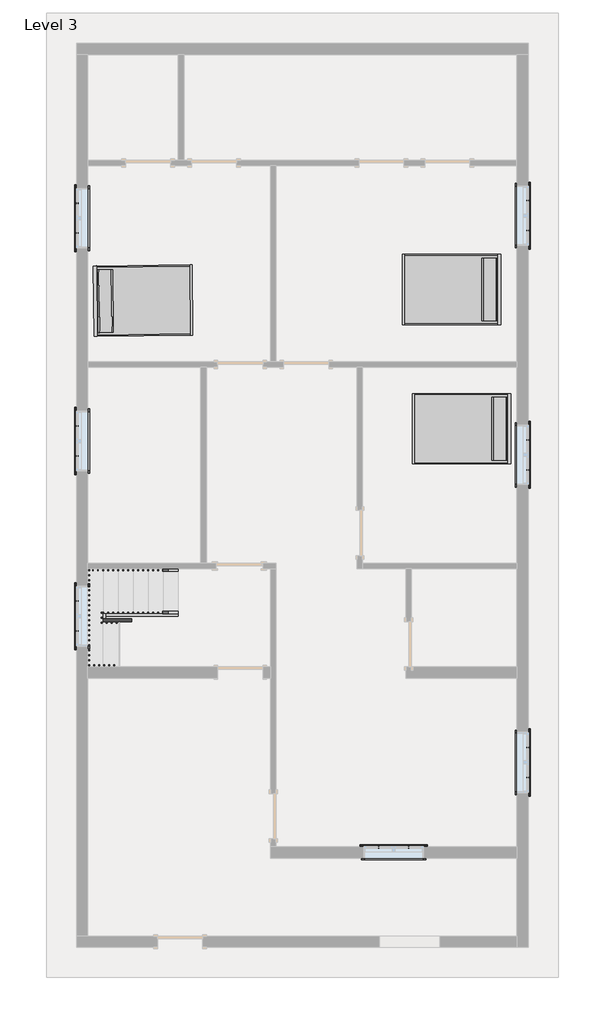
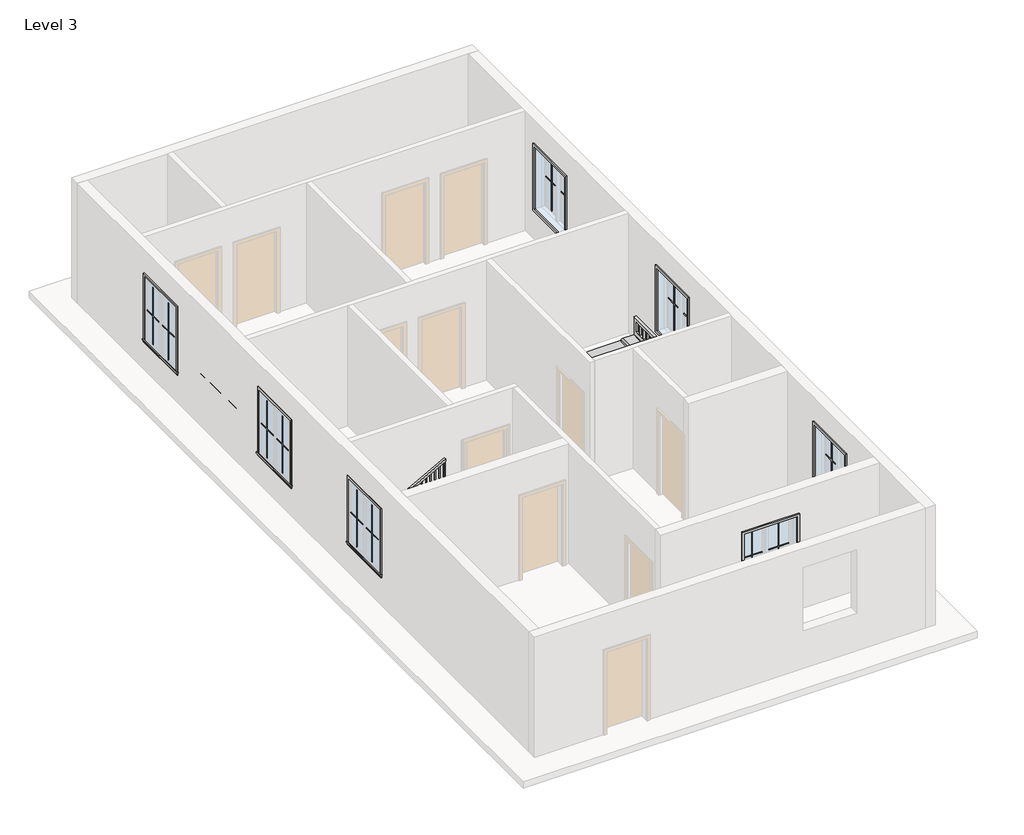
# One storey, part 2 of 2: 28 proxies, 3 furniture elements, 3 members, 2 railings.
"""IFC4 building model written with IfcOpenShell, lengths in millimetres."""

from ifc_helpers import new_model, si_unit, frame, origin, place, context, project, spatial, polyline, outline, extrude, faceted_brep, transform, mapped, element, save
from components import muntin_pattern_2x2_muntin_pattern_2x2_6dad3731, muntin_pattern_2x2_muntin_pattern_2x2_a30a3345, trim_window_exterior_flat_with_sill_92b9b949, trim_window_interior_flat_picture_frame_3bb882cf, furniture_121fd3aa

model = new_model("IFC4")

# Units and contexts
model_context = context("Model", 3, world=origin())
ifc_project = project(units=[si_unit("LENGTHUNIT", "METRE", prefix="MILLI")], contexts=[model_context])

# Site, building, storey
site = spatial("IfcSite", under=ifc_project)
building = spatial("IfcBuilding", under=site)
storey = spatial("IfcBuildingStorey", under=building, Name="Level 3", Elevation=6096.0)

# Proxies
placement = place(None, origin())
muntin_pattern_2x2_muntin_pattern_2x2_shape = muntin_pattern_2x2_muntin_pattern_2x2_6dad3731(model_context)
element("IfcBuildingElementProxy", 1, Name="Muntin Pattern_2x2 : Muntin Pattern_2x2", ObjectType="Muntin Pattern_2x2 : Muntin Pattern_2x2", at=placement, inside=storey, context=model_context, shape_type="MappedRepresentation", body=[
    mapped(muntin_pattern_2x2_muntin_pattern_2x2_shape, transform((1279.525, 5621.3375, 7080.25), x_axis=(0.0, 1.0, 0.0), y_axis=(-1.0, 0.0, 0.0), z_axis=(0.0, 0.0, 1.0))),
])
element("IfcBuildingElementProxy", 2, Name="Muntin Pattern_2x2 : Muntin Pattern_2x2", ObjectType="Muntin Pattern_2x2 : Muntin Pattern_2x2", at=placement, inside=storey, context=model_context, shape_type="MappedRepresentation", body=[
    mapped(muntin_pattern_2x2_muntin_pattern_2x2_shape, transform((1279.525, 10129.8375, 7080.25), x_axis=(0.0, 1.0, 0.0), y_axis=(-1.0, 0.0, 0.0), z_axis=(0.0, 0.0, 1.0))),
])
element("IfcBuildingElementProxy", 3, Name="Muntin Pattern_2x2 : Muntin Pattern_2x2", ObjectType="Muntin Pattern_2x2 : Muntin Pattern_2x2", at=placement, inside=storey, context=model_context, shape_type="MappedRepresentation", body=[
    mapped(muntin_pattern_2x2_muntin_pattern_2x2_shape, transform((10404.475, 10787.0625, 7080.25), x_axis=(0.0, -1.0, 0.0), y_axis=(1.0, 0.0, 0.0), z_axis=(0.0, 0.0, 1.0))),
])
element("IfcBuildingElementProxy", 4, Name="Muntin Pattern_2x2 : Muntin Pattern_2x2", ObjectType="Muntin Pattern_2x2 : Muntin Pattern_2x2", at=placement, inside=storey, context=model_context, shape_type="MappedRepresentation", body=[
    mapped(muntin_pattern_2x2_muntin_pattern_2x2_shape, transform((10404.475, 5948.3625, 7080.25), x_axis=(0.0, -1.0, 0.0), y_axis=(1.0, 0.0, 0.0), z_axis=(0.0, 0.0, 1.0))),
])
element("IfcBuildingElementProxy", 5, Name="Muntin Pattern_2x2 : Muntin Pattern_2x2", ObjectType="Muntin Pattern_2x2 : Muntin Pattern_2x2", at=placement, inside=storey, context=model_context, shape_type="MappedRepresentation", body=[
    mapped(muntin_pattern_2x2_muntin_pattern_2x2_shape, transform((10404.475, -274.6375, 7080.25), x_axis=(0.0, -1.0, 0.0), y_axis=(1.0, 0.0, 0.0), z_axis=(0.0, 0.0, 1.0))),
])
element("IfcBuildingElementProxy", 6, Name="Muntin Pattern_2x2 : Muntin Pattern_2x2", ObjectType="Muntin Pattern_2x2 : Muntin Pattern_2x2", at=placement, inside=storey, context=model_context, shape_type="MappedRepresentation", body=[
    mapped(muntin_pattern_2x2_muntin_pattern_2x2_shape, transform((7386.6375, -2295.525, 7080.25), x_axis=(1.0, 0.0, 0.0), y_axis=(0.0, 1.0, 0.0), z_axis=(0.0, 0.0, 1.0))),
])
element("IfcBuildingElementProxy", 7, Name="Muntin Pattern_2x2 : Muntin Pattern_2x2", ObjectType="Muntin Pattern_2x2 : Muntin Pattern_2x2", at=placement, inside=storey, context=model_context, shape_type="MappedRepresentation", body=[
    mapped(muntin_pattern_2x2_muntin_pattern_2x2_shape, transform((1279.525, 2078.0375, 7080.25), x_axis=(0.0, 1.0, 0.0), y_axis=(-1.0, 0.0, 0.0), z_axis=(0.0, 0.0, 1.0))),
])
muntin_pattern_2x2_muntin_pattern_2x2_2_shape = muntin_pattern_2x2_muntin_pattern_2x2_a30a3345(model_context)
element("IfcBuildingElementProxy", 8, Name="Muntin Pattern_2x2 : Muntin Pattern_2x2", ObjectType="Muntin Pattern_2x2 : Muntin Pattern_2x2", at=placement, inside=storey, context=model_context, shape_type="MappedRepresentation", body=[
    mapped(muntin_pattern_2x2_muntin_pattern_2x2_2_shape, transform((1279.525, 6227.7625, 7080.25), x_axis=(0.0, -1.0, 0.0), y_axis=(1.0, 0.0, 0.0), z_axis=(0.0, 0.0, 1.0))),
])
element("IfcBuildingElementProxy", 9, Name="Muntin Pattern_2x2 : Muntin Pattern_2x2", ObjectType="Muntin Pattern_2x2 : Muntin Pattern_2x2", at=placement, inside=storey, context=model_context, shape_type="MappedRepresentation", body=[
    mapped(muntin_pattern_2x2_muntin_pattern_2x2_2_shape, transform((1279.525, 10736.2625, 7080.25), x_axis=(0.0, -1.0, 0.0), y_axis=(1.0, 0.0, 0.0), z_axis=(0.0, 0.0, 1.0))),
])
element("IfcBuildingElementProxy", 10, Name="Muntin Pattern_2x2 : Muntin Pattern_2x2", ObjectType="Muntin Pattern_2x2 : Muntin Pattern_2x2", at=placement, inside=storey, context=model_context, shape_type="MappedRepresentation", body=[
    mapped(muntin_pattern_2x2_muntin_pattern_2x2_2_shape, transform((10404.475, 10180.6375, 7080.25), x_axis=(0.0, 1.0, 0.0), y_axis=(-1.0, 0.0, 0.0), z_axis=(0.0, 0.0, 1.0))),
])
element("IfcBuildingElementProxy", 11, Name="Muntin Pattern_2x2 : Muntin Pattern_2x2", ObjectType="Muntin Pattern_2x2 : Muntin Pattern_2x2", at=placement, inside=storey, context=model_context, shape_type="MappedRepresentation", body=[
    mapped(muntin_pattern_2x2_muntin_pattern_2x2_2_shape, transform((10404.475, 5341.9375, 7080.25), x_axis=(0.0, 1.0, 0.0), y_axis=(-1.0, 0.0, 0.0), z_axis=(0.0, 0.0, 1.0))),
])
element("IfcBuildingElementProxy", 12, Name="Muntin Pattern_2x2 : Muntin Pattern_2x2", ObjectType="Muntin Pattern_2x2 : Muntin Pattern_2x2", at=placement, inside=storey, context=model_context, shape_type="MappedRepresentation", body=[
    mapped(muntin_pattern_2x2_muntin_pattern_2x2_2_shape, transform((10404.475, -881.0625, 7080.25), x_axis=(0.0, 1.0, 0.0), y_axis=(-1.0, 0.0, 0.0), z_axis=(0.0, 0.0, 1.0))),
])
element("IfcBuildingElementProxy", 13, Name="Muntin Pattern_2x2 : Muntin Pattern_2x2", ObjectType="Muntin Pattern_2x2 : Muntin Pattern_2x2", at=placement, inside=storey, context=model_context, shape_type="MappedRepresentation", body=[
    mapped(muntin_pattern_2x2_muntin_pattern_2x2_2_shape, transform((7993.0625, -2295.525, 7080.25), x_axis=(-1.0, 0.0, 0.0), y_axis=(0.0, -1.0, 0.0), z_axis=(0.0, 0.0, 1.0))),
])
element("IfcBuildingElementProxy", 14, Name="Muntin Pattern_2x2 : Muntin Pattern_2x2", ObjectType="Muntin Pattern_2x2 : Muntin Pattern_2x2", at=placement, inside=storey, context=model_context, shape_type="MappedRepresentation", body=[
    mapped(muntin_pattern_2x2_muntin_pattern_2x2_2_shape, transform((1279.525, 2684.4625, 7080.25), x_axis=(0.0, -1.0, 0.0), y_axis=(1.0, 0.0, 0.0), z_axis=(0.0, 0.0, 1.0))),
])
trim_window_exterior_flat_with_sill_shape = trim_window_exterior_flat_with_sill_92b9b949(model_context)
element("IfcBuildingElementProxy", 15, Name="Trim-Window-Exterior-Flat : with Sill", ObjectType="Trim-Window-Exterior-Flat : with Sill", at=placement, inside=storey, context=model_context, shape_type="MappedRepresentation", body=[
    mapped(trim_window_exterior_flat_with_sill_shape, transform((1270.0, 5924.55, 8534.4), x_axis=(0.0, -1.0, 0.0), y_axis=(0.0, 0.0, 1.0), z_axis=(-1.0, 0.0, 0.0))),
])
element("IfcBuildingElementProxy", 16, Name="Trim-Window-Exterior-Flat : with Sill", ObjectType="Trim-Window-Exterior-Flat : with Sill", at=placement, inside=storey, context=model_context, shape_type="MappedRepresentation", body=[
    mapped(trim_window_exterior_flat_with_sill_shape, transform((1270.0, 10433.05, 8534.4), x_axis=(0.0, -1.0, 0.0), y_axis=(0.0, 0.0, 1.0), z_axis=(-1.0, 0.0, 0.0))),
])
element("IfcBuildingElementProxy", 17, Name="Trim-Window-Exterior-Flat : with Sill", ObjectType="Trim-Window-Exterior-Flat : with Sill", at=placement, inside=storey, context=model_context, shape_type="MappedRepresentation", body=[
    mapped(trim_window_exterior_flat_with_sill_shape, transform((10414.0, 10483.85, 8534.4), x_axis=(0.0, 1.0, 0.0), y_axis=(0.0, 0.0, 1.0), z_axis=(1.0, 0.0, 0.0))),
])
element("IfcBuildingElementProxy", 18, Name="Trim-Window-Exterior-Flat : with Sill", ObjectType="Trim-Window-Exterior-Flat : with Sill", at=placement, inside=storey, context=model_context, shape_type="MappedRepresentation", body=[
    mapped(trim_window_exterior_flat_with_sill_shape, transform((10414.0, 5645.15, 8534.4), x_axis=(0.0, 1.0, 0.0), y_axis=(0.0, 0.0, 1.0), z_axis=(1.0, 0.0, 0.0))),
])
element("IfcBuildingElementProxy", 19, Name="Trim-Window-Exterior-Flat : with Sill", ObjectType="Trim-Window-Exterior-Flat : with Sill", at=placement, inside=storey, context=model_context, shape_type="MappedRepresentation", body=[
    mapped(trim_window_exterior_flat_with_sill_shape, transform((10414.0, -577.85, 8534.4), x_axis=(0.0, 1.0, 0.0), y_axis=(0.0, 0.0, 1.0), z_axis=(1.0, 0.0, 0.0))),
])
element("IfcBuildingElementProxy", 20, Name="Trim-Window-Exterior-Flat : with Sill", ObjectType="Trim-Window-Exterior-Flat : with Sill", at=placement, inside=storey, context=model_context, shape_type="MappedRepresentation", body=[
    mapped(trim_window_exterior_flat_with_sill_shape, transform((7689.85, -2286.0, 8534.4), x_axis=(-1.0, 0.0, 0.0), y_axis=(0.0, 0.0, 1.0), z_axis=(0.0, 1.0, 0.0))),
])
element("IfcBuildingElementProxy", 21, Name="Trim-Window-Exterior-Flat : with Sill", ObjectType="Trim-Window-Exterior-Flat : with Sill", at=placement, inside=storey, context=model_context, shape_type="MappedRepresentation", body=[
    mapped(trim_window_exterior_flat_with_sill_shape, transform((1270.0, 2381.25, 8534.4), x_axis=(0.0, -1.0, 0.0), y_axis=(0.0, 0.0, 1.0), z_axis=(-1.0, 0.0, 0.0))),
])
trim_window_interior_flat_picture_frame_shape = trim_window_interior_flat_picture_frame_3bb882cf(model_context)
element("IfcBuildingElementProxy", 22, Name="Trim-Window-Interior-Flat : Picture Frame", ObjectType="Trim-Window-Interior-Flat : Picture Frame", at=placement, inside=storey, context=model_context, shape_type="MappedRepresentation", body=[
    mapped(trim_window_interior_flat_picture_frame_shape, transform((1498.6, 5924.55, 8534.4), x_axis=(0.0, 1.0, 0.0), y_axis=(0.0, 0.0, 1.0), z_axis=(1.0, 0.0, 0.0))),
])
element("IfcBuildingElementProxy", 23, Name="Trim-Window-Interior-Flat : Picture Frame", ObjectType="Trim-Window-Interior-Flat : Picture Frame", at=placement, inside=storey, context=model_context, shape_type="MappedRepresentation", body=[
    mapped(trim_window_interior_flat_picture_frame_shape, transform((1498.6, 10433.05, 8534.4), x_axis=(0.0, 1.0, 0.0), y_axis=(0.0, 0.0, 1.0), z_axis=(1.0, 0.0, 0.0))),
])
element("IfcBuildingElementProxy", 24, Name="Trim-Window-Interior-Flat : Picture Frame", ObjectType="Trim-Window-Interior-Flat : Picture Frame", at=placement, inside=storey, context=model_context, shape_type="MappedRepresentation", body=[
    mapped(trim_window_interior_flat_picture_frame_shape, transform((10185.4, 10483.85, 8534.4), x_axis=(0.0, -1.0, 0.0), y_axis=(0.0, 0.0, 1.0), z_axis=(-1.0, 0.0, 0.0))),
])
element("IfcBuildingElementProxy", 25, Name="Trim-Window-Interior-Flat : Picture Frame", ObjectType="Trim-Window-Interior-Flat : Picture Frame", at=placement, inside=storey, context=model_context, shape_type="MappedRepresentation", body=[
    mapped(trim_window_interior_flat_picture_frame_shape, transform((10185.4, 5645.15, 8534.4), x_axis=(0.0, -1.0, 0.0), y_axis=(0.0, 0.0, 1.0), z_axis=(-1.0, 0.0, 0.0))),
])
element("IfcBuildingElementProxy", 26, Name="Trim-Window-Interior-Flat : Picture Frame", ObjectType="Trim-Window-Interior-Flat : Picture Frame", at=placement, inside=storey, context=model_context, shape_type="MappedRepresentation", body=[
    mapped(trim_window_interior_flat_picture_frame_shape, transform((10185.4, -577.85, 8534.4), x_axis=(0.0, -1.0, 0.0), y_axis=(0.0, 0.0, 1.0), z_axis=(-1.0, 0.0, 0.0))),
])
element("IfcBuildingElementProxy", 27, Name="Trim-Window-Interior-Flat : Picture Frame", ObjectType="Trim-Window-Interior-Flat : Picture Frame", at=placement, inside=storey, context=model_context, shape_type="MappedRepresentation", body=[
    mapped(trim_window_interior_flat_picture_frame_shape, transform((7689.85, -2514.6, 8534.4), x_axis=(1.0, 0.0, 0.0), y_axis=(0.0, 0.0, 1.0), z_axis=(0.0, -1.0, 0.0))),
])
element("IfcBuildingElementProxy", 28, Name="Trim-Window-Interior-Flat : Picture Frame", ObjectType="Trim-Window-Interior-Flat : Picture Frame", at=placement, inside=storey, context=model_context, shape_type="MappedRepresentation", body=[
    mapped(trim_window_interior_flat_picture_frame_shape, transform((1498.6, 2381.25, 8534.4), x_axis=(0.0, 1.0, 0.0), y_axis=(0.0, 0.0, 1.0), z_axis=(1.0, 0.0, 0.0))),
])

# Furniture
furniture_shape = furniture_121fd3aa(model_context)
element("IfcFurniture", 29, ObjectType="Bed-Shaker : Double 56\" x 78\"", at=placement, inside=storey, context=model_context, shape_type="MappedRepresentation", body=[
    mapped(furniture_shape, transform((9849.8308516, 8970.3536289, 6096.0), x_axis=(0.0, -1.0, 0.0), y_axis=(1.0, 0.0, 0.0), z_axis=(0.0, 0.0, 1.0))),
])
element("IfcFurniture", 30, ObjectType="Bed-Shaker : Double 56\" x 78\"", at=placement, inside=storey, context=model_context, shape_type="MappedRepresentation", body=[
    mapped(furniture_shape, transform((10050.5002502, 6155.12029, 6096.0), x_axis=(0.0, -1.0, 0.0), y_axis=(1.0, 0.0, 0.0), z_axis=(0.0, 0.0, 1.0))),
])
element("IfcFurniture", 31, ObjectType="Bed-Shaker : Double 56\" x 78\"", at=placement, inside=storey, context=model_context, shape_type="MappedRepresentation", body=[
    mapped(furniture_shape, transform((1630.8006063, 8772.9712322, 6096.0), x_axis=(-0.01124472055544287, 0.9999367761311863, 0.0), y_axis=(-0.9999367761311863, -0.01124472055544287, 0.0), z_axis=(0.0, 0.0, 1.0))),
])

# Members
element("IfcMember", 32, ObjectType="Stringer - 2\" Width", at=placement, inside=storey, context=model_context, shape_type="SweptSolid", body=[
    extrude(outline(polyline([(6096.0, 3327.4), (6303.5983948, 3327.4), (7122.0428392, 1854.2), (6773.3641651, 1854.2), (6096.0, 3073.4554972), (6096.0, 3327.4)])), frame((0.0, 2374.9, 0.0), z_axis=(0.0, 1.0, 0.0), x_axis=(0.0, 0.0, 1.0)), (0.0, 0.0, 1.0), 50.8),
])
element("IfcMember", 33, ObjectType="Stringer - 2\" Width", at=placement, inside=storey, context=model_context, shape_type="SweptSolid", body=[
    extrude(outline(polyline([(1803.4, 2425.7), (1854.2, 2425.7), (1854.2, 2324.1), (1803.4, 2324.1), (1803.4, 2425.7)])), frame((0.0, 0.0, 6883.4), z_axis=(0.0, 0.0, 1.0), x_axis=(1.0, 0.0, 0.0)), (0.0, 0.0, 1.0), 304.8),
])
element("IfcMember", 34, ObjectType="Stringer - 2\" Width", at=placement, inside=storey, context=model_context, shape_type="SweptSolid", body=[
    extrude(outline(polyline([(7319.5983948, 1803.4), (6970.9197207, 1803.4), (7648.253054, 3022.6), (7996.9317281, 3022.6), (7319.5983948, 1803.4)])), frame((0.0, 2273.3, 0.0), z_axis=(0.0, 1.0, 0.0), x_axis=(0.0, 0.0, 1.0)), (0.0, 0.0, 1.0), 50.8),
])

# Railings
element("IfcRailing", 35, ObjectType="Handrail - Rectangular", at=placement, inside=storey, context=model_context, shape_type="SolidModel", body=[
    faceted_brep([(3327.4, 3289.3, 7179.7333333), (3327.4, 3289.3, 7121.620221), (3327.4, 3340.1, 7121.620221), (3327.4, 3340.1, 7179.7333333), (1803.4, 3289.3, 8026.4), (1790.2363978, 3289.3, 7975.6), (1790.2363978, 3340.1, 7975.6), (1803.4, 3340.1, 8026.4), (1549.4, 3289.3, 8026.4), (1549.4, 3289.3, 7975.6), (1498.6, 3340.1, 7975.6), (1498.6, 3340.1, 8026.4), (1549.4, 1485.9, 8026.4), (1549.4, 1435.1, 7975.6), (1498.6, 1435.1, 7975.6), (1498.6, 1485.9, 8026.4), (1549.4, 1485.9, 8096.9555556), (1549.4, 1435.1, 8046.1555556), (1498.6, 1435.1, 8046.1555556), (1498.6, 1485.9, 8096.9555556), (1549.4, 1409.7, 8096.9555556), (1549.4, 1409.7, 8046.1555556), (1498.6, 1358.9, 8046.1555556), (1498.6, 1358.9, 8096.9555556), (1625.6, 1409.7, 8096.9555556), (1638.7636022, 1409.7, 8046.1555556), (1638.7636022, 1358.9, 8046.1555556), (1625.6, 1358.9, 8096.9555556), (3022.6, 1409.7, 8873.0666667), (3022.6, 1358.9, 8873.0666667), (3022.6, 1358.9, 8814.9535543), (3022.6, 1409.7, 8814.9535543)], [[[0, 1, 2, 3]], [[1, 0, 4, 5]], [[2, 1, 5, 6]], [[3, 2, 6, 7]], [[0, 3, 7, 4]], [[5, 4, 8, 9]], [[6, 5, 9, 10]], [[7, 6, 10, 11]], [[4, 7, 11, 8]], [[9, 8, 12, 13]], [[10, 9, 13, 14]], [[11, 10, 14, 15]], [[8, 11, 15, 12]], [[13, 12, 16, 17]], [[14, 13, 17, 18]], [[15, 14, 18, 19]], [[12, 15, 19, 16]], [[17, 16, 20, 21]], [[18, 17, 21, 22]], [[19, 18, 22, 23]], [[16, 19, 23, 20]], [[21, 20, 24, 25]], [[22, 21, 25, 26]], [[23, 22, 26, 27]], [[20, 23, 27, 24]], [[28, 29, 30, 31]], [[25, 24, 28, 31]], [[26, 25, 31, 30]], [[27, 26, 30, 29]], [[24, 27, 29, 28]]]),
    extrude(outline(polyline([(8777.9118876, 2955.925), (8767.3285543, 2936.875), (7789.3333333, 2936.875), (7789.3333333, 2955.925), (8777.9118876, 2955.925)])), frame((0.0, 1374.775, 0.0), z_axis=(0.0, 1.0, 0.0), x_axis=(0.0, 0.0, 1.0)), (0.0, 0.0, 1.0), 19.05),
    extrude(outline(polyline([(8721.4674432, 2854.325), (8710.8841099, 2835.275), (7789.3333333, 2835.275), (7789.3333333, 2854.325), (8721.4674432, 2854.325)])), frame((0.0, 1374.775, 0.0), z_axis=(0.0, 1.0, 0.0), x_axis=(0.0, 0.0, 1.0)), (0.0, 0.0, 1.0), 19.05),
    extrude(outline(polyline([(8665.0229988, 2752.725), (8654.4396654, 2733.675), (7789.3333333, 2733.675), (7789.3333333, 2752.725), (8665.0229988, 2752.725)])), frame((0.0, 1374.775, 0.0), z_axis=(0.0, 1.0, 0.0), x_axis=(0.0, 0.0, 1.0)), (0.0, 0.0, 1.0), 19.05),
    extrude(outline(polyline([(8608.5785543, 2651.125), (8597.995221, 2632.075), (7620.0, 2632.075), (7620.0, 2651.125), (8608.5785543, 2651.125)])), frame((0.0, 1374.775, 0.0), z_axis=(0.0, 1.0, 0.0), x_axis=(0.0, 0.0, 1.0)), (0.0, 0.0, 1.0), 19.05),
    extrude(outline(polyline([(8552.1341099, 2549.525), (8541.5507765, 2530.475), (7620.0, 2530.475), (7620.0, 2549.525), (8552.1341099, 2549.525)])), frame((0.0, 1374.775, 0.0), z_axis=(0.0, 1.0, 0.0), x_axis=(0.0, 0.0, 1.0)), (0.0, 0.0, 1.0), 19.05),
    extrude(outline(polyline([(8495.6896654, 2447.925), (8485.1063321, 2428.875), (7620.0, 2428.875), (7620.0, 2447.925), (8495.6896654, 2447.925)])), frame((0.0, 1374.775, 0.0), z_axis=(0.0, 1.0, 0.0), x_axis=(0.0, 0.0, 1.0)), (0.0, 0.0, 1.0), 19.05),
    extrude(outline(polyline([(8439.245221, 2346.325), (8428.6618876, 2327.275), (7450.6666667, 2327.275), (7450.6666667, 2346.325), (8439.245221, 2346.325)])), frame((0.0, 1374.775, 0.0), z_axis=(0.0, 1.0, 0.0), x_axis=(0.0, 0.0, 1.0)), (0.0, 0.0, 1.0), 19.05),
    extrude(outline(polyline([(8382.8007765, 2244.725), (8372.2174432, 2225.675), (7450.6666667, 2225.675), (7450.6666667, 2244.725), (8382.8007765, 2244.725)])), frame((0.0, 1374.775, 0.0), z_axis=(0.0, 1.0, 0.0), x_axis=(0.0, 0.0, 1.0)), (0.0, 0.0, 1.0), 19.05),
    extrude(outline(polyline([(8326.3563321, 2143.125), (8315.7729988, 2124.075), (7450.6666667, 2124.075), (7450.6666667, 2143.125), (8326.3563321, 2143.125)])), frame((0.0, 1374.775, 0.0), z_axis=(0.0, 1.0, 0.0), x_axis=(0.0, 0.0, 1.0)), (0.0, 0.0, 1.0), 19.05),
    extrude(outline(polyline([(8269.9118876, 2041.525), (8259.3285543, 2022.475), (7281.3333333, 2022.475), (7281.3333333, 2041.525), (8269.9118876, 2041.525)])), frame((0.0, 1374.775, 0.0), z_axis=(0.0, 1.0, 0.0), x_axis=(0.0, 0.0, 1.0)), (0.0, 0.0, 1.0), 19.05),
    extrude(outline(polyline([(8213.4674432, 1939.925), (8202.8841099, 1920.875), (7281.3333333, 1920.875), (7281.3333333, 1939.925), (8213.4674432, 1939.925)])), frame((0.0, 1374.775, 0.0), z_axis=(0.0, 1.0, 0.0), x_axis=(0.0, 0.0, 1.0)), (0.0, 0.0, 1.0), 19.05),
    extrude(outline(polyline([(8157.0229988, 1838.325), (8146.4396654, 1819.275), (7281.3333333, 1819.275), (7281.3333333, 1838.325), (8157.0229988, 1838.325)])), frame((0.0, 1374.775, 0.0), z_axis=(0.0, 1.0, 0.0), x_axis=(0.0, 0.0, 1.0)), (0.0, 0.0, 1.0), 19.05),
    extrude(outline(polyline([(8100.5785543, 1736.725), (8089.995221, 1717.675), (7112.0, 1717.675), (7112.0, 1736.725), (8100.5785543, 1736.725)])), frame((0.0, 1374.775, 0.0), z_axis=(0.0, 1.0, 0.0), x_axis=(0.0, 0.0, 1.0)), (0.0, 0.0, 1.0), 19.05),
    extrude(outline(polyline([(8044.1341099, 1635.125), (8033.5507765, 1616.075), (7112.0, 1616.075), (7112.0, 1635.125), (8044.1341099, 1635.125)])), frame((0.0, 1374.775, 0.0), z_axis=(0.0, 1.0, 0.0), x_axis=(0.0, 0.0, 1.0)), (0.0, 0.0, 1.0), 19.05),
    extrude(outline(polyline([(1514.475, 1495.425), (1533.525, 1495.425), (1533.525, 1476.375), (1514.475, 1476.375), (1514.475, 1495.425)])), frame((0.0, 0.0, 7112.0), z_axis=(0.0, 0.0, 1.0), x_axis=(1.0, 0.0, 0.0)), (0.0, 0.0, 1.0), 863.6),
    extrude(outline(polyline([(1514.475, 1597.025), (1533.525, 1597.025), (1533.525, 1577.975), (1514.475, 1577.975), (1514.475, 1597.025)])), frame((0.0, 0.0, 7112.0), z_axis=(0.0, 0.0, 1.0), x_axis=(1.0, 0.0, 0.0)), (0.0, 0.0, 1.0), 863.6),
    extrude(outline(polyline([(1514.475, 1698.625), (1533.525, 1698.625), (1533.525, 1679.575), (1514.475, 1679.575), (1514.475, 1698.625)])), frame((0.0, 0.0, 7112.0), z_axis=(0.0, 0.0, 1.0), x_axis=(1.0, 0.0, 0.0)), (0.0, 0.0, 1.0), 863.6),
    extrude(outline(polyline([(1514.475, 1800.225), (1533.525, 1800.225), (1533.525, 1781.175), (1514.475, 1781.175), (1514.475, 1800.225)])), frame((0.0, 0.0, 7112.0), z_axis=(0.0, 0.0, 1.0), x_axis=(1.0, 0.0, 0.0)), (0.0, 0.0, 1.0), 863.6),
    extrude(outline(polyline([(1514.475, 1901.825), (1533.525, 1901.825), (1533.525, 1882.775), (1514.475, 1882.775), (1514.475, 1901.825)])), frame((0.0, 0.0, 7112.0), z_axis=(0.0, 0.0, 1.0), x_axis=(1.0, 0.0, 0.0)), (0.0, 0.0, 1.0), 863.6),
    extrude(outline(polyline([(1514.475, 2003.425), (1533.525, 2003.425), (1533.525, 1984.375), (1514.475, 1984.375), (1514.475, 2003.425)])), frame((0.0, 0.0, 7112.0), z_axis=(0.0, 0.0, 1.0), x_axis=(1.0, 0.0, 0.0)), (0.0, 0.0, 1.0), 863.6),
    extrude(outline(polyline([(1514.475, 2105.025), (1533.525, 2105.025), (1533.525, 2085.975), (1514.475, 2085.975), (1514.475, 2105.025)])), frame((0.0, 0.0, 7112.0), z_axis=(0.0, 0.0, 1.0), x_axis=(1.0, 0.0, 0.0)), (0.0, 0.0, 1.0), 863.6),
    extrude(outline(polyline([(1514.475, 2206.625), (1533.525, 2206.625), (1533.525, 2187.575), (1514.475, 2187.575), (1514.475, 2206.625)])), frame((0.0, 0.0, 7112.0), z_axis=(0.0, 0.0, 1.0), x_axis=(1.0, 0.0, 0.0)), (0.0, 0.0, 1.0), 863.6),
    extrude(outline(polyline([(1514.475, 2308.225), (1533.525, 2308.225), (1533.525, 2289.175), (1514.475, 2289.175), (1514.475, 2308.225)])), frame((0.0, 0.0, 7112.0), z_axis=(0.0, 0.0, 1.0), x_axis=(1.0, 0.0, 0.0)), (0.0, 0.0, 1.0), 863.6),
    extrude(outline(polyline([(1514.475, 2409.825), (1533.525, 2409.825), (1533.525, 2390.775), (1514.475, 2390.775), (1514.475, 2409.825)])), frame((0.0, 0.0, 7112.0), z_axis=(0.0, 0.0, 1.0), x_axis=(1.0, 0.0, 0.0)), (0.0, 0.0, 1.0), 863.6),
    extrude(outline(polyline([(1514.475, 2511.425), (1533.525, 2511.425), (1533.525, 2492.375), (1514.475, 2492.375), (1514.475, 2511.425)])), frame((0.0, 0.0, 7112.0), z_axis=(0.0, 0.0, 1.0), x_axis=(1.0, 0.0, 0.0)), (0.0, 0.0, 1.0), 863.6),
    extrude(outline(polyline([(1514.475, 2613.025), (1533.525, 2613.025), (1533.525, 2593.975), (1514.475, 2593.975), (1514.475, 2613.025)])), frame((0.0, 0.0, 7112.0), z_axis=(0.0, 0.0, 1.0), x_axis=(1.0, 0.0, 0.0)), (0.0, 0.0, 1.0), 863.6),
    extrude(outline(polyline([(1514.475, 2714.625), (1533.525, 2714.625), (1533.525, 2695.575), (1514.475, 2695.575), (1514.475, 2714.625)])), frame((0.0, 0.0, 7112.0), z_axis=(0.0, 0.0, 1.0), x_axis=(1.0, 0.0, 0.0)), (0.0, 0.0, 1.0), 863.6),
    extrude(outline(polyline([(1514.475, 2816.225), (1533.525, 2816.225), (1533.525, 2797.175), (1514.475, 2797.175), (1514.475, 2816.225)])), frame((0.0, 0.0, 7112.0), z_axis=(0.0, 0.0, 1.0), x_axis=(1.0, 0.0, 0.0)), (0.0, 0.0, 1.0), 863.6),
    extrude(outline(polyline([(1514.475, 2917.825), (1533.525, 2917.825), (1533.525, 2898.775), (1514.475, 2898.775), (1514.475, 2917.825)])), frame((0.0, 0.0, 7112.0), z_axis=(0.0, 0.0, 1.0), x_axis=(1.0, 0.0, 0.0)), (0.0, 0.0, 1.0), 863.6),
    extrude(outline(polyline([(1514.475, 3019.425), (1533.525, 3019.425), (1533.525, 3000.375), (1514.475, 3000.375), (1514.475, 3019.425)])), frame((0.0, 0.0, 7112.0), z_axis=(0.0, 0.0, 1.0), x_axis=(1.0, 0.0, 0.0)), (0.0, 0.0, 1.0), 863.6),
    extrude(outline(polyline([(1514.475, 3121.025), (1533.525, 3121.025), (1533.525, 3101.975), (1514.475, 3101.975), (1514.475, 3121.025)])), frame((0.0, 0.0, 7112.0), z_axis=(0.0, 0.0, 1.0), x_axis=(1.0, 0.0, 0.0)), (0.0, 0.0, 1.0), 863.6),
    extrude(outline(polyline([(1514.475, 3222.625), (1533.525, 3222.625), (1533.525, 3203.575), (1514.475, 3203.575), (1514.475, 3222.625)])), frame((0.0, 0.0, 7112.0), z_axis=(0.0, 0.0, 1.0), x_axis=(1.0, 0.0, 0.0)), (0.0, 0.0, 1.0), 863.6),
    extrude(outline(polyline([(1609.725, 3324.225), (1609.725, 3305.175), (1590.675, 3305.175), (1590.675, 3324.225), (1609.725, 3324.225)])), frame((0.0, 0.0, 7112.0), z_axis=(0.0, 0.0, 1.0), x_axis=(1.0, 0.0, 0.0)), (0.0, 0.0, 1.0), 863.6),
    extrude(outline(polyline([(1711.325, 3324.225), (1711.325, 3305.175), (1692.275, 3305.175), (1692.275, 3324.225), (1711.325, 3324.225)])), frame((0.0, 0.0, 7112.0), z_axis=(0.0, 0.0, 1.0), x_axis=(1.0, 0.0, 0.0)), (0.0, 0.0, 1.0), 863.6),
    extrude(outline(polyline([(7962.995221, 1812.925), (7973.5785543, 1793.875), (7112.0, 1793.875), (7112.0, 1812.925), (7962.995221, 1812.925)])), frame((0.0, 3305.175, 0.0), z_axis=(0.0, 1.0, 0.0), x_axis=(0.0, 0.0, 1.0)), (0.0, 0.0, 1.0), 19.05),
    extrude(outline(polyline([(7906.5507765, 1914.525), (7917.1341099, 1895.475), (6942.6666667, 1895.475), (6942.6666667, 1914.525), (7906.5507765, 1914.525)])), frame((0.0, 3305.175, 0.0), z_axis=(0.0, 1.0, 0.0), x_axis=(0.0, 0.0, 1.0)), (0.0, 0.0, 1.0), 19.05),
    extrude(outline(polyline([(7850.1063321, 2016.125), (7860.6896654, 1997.075), (6942.6666667, 1997.075), (6942.6666667, 2016.125), (7850.1063321, 2016.125)])), frame((0.0, 3305.175, 0.0), z_axis=(0.0, 1.0, 0.0), x_axis=(0.0, 0.0, 1.0)), (0.0, 0.0, 1.0), 19.05),
    extrude(outline(polyline([(7793.6618876, 2117.725), (7804.245221, 2098.675), (6942.6666667, 2098.675), (6942.6666667, 2117.725), (7793.6618876, 2117.725)])), frame((0.0, 3305.175, 0.0), z_axis=(0.0, 1.0, 0.0), x_axis=(0.0, 0.0, 1.0)), (0.0, 0.0, 1.0), 19.05),
    extrude(outline(polyline([(7737.2174432, 2219.325), (7747.8007765, 2200.275), (6773.3333333, 2200.275), (6773.3333333, 2219.325), (7737.2174432, 2219.325)])), frame((0.0, 3305.175, 0.0), z_axis=(0.0, 1.0, 0.0), x_axis=(0.0, 0.0, 1.0)), (0.0, 0.0, 1.0), 19.05),
    extrude(outline(polyline([(7680.7729988, 2320.925), (7691.3563321, 2301.875), (6773.3333333, 2301.875), (6773.3333333, 2320.925), (7680.7729988, 2320.925)])), frame((0.0, 3305.175, 0.0), z_axis=(0.0, 1.0, 0.0), x_axis=(0.0, 0.0, 1.0)), (0.0, 0.0, 1.0), 19.05),
    extrude(outline(polyline([(7624.3285543, 2422.525), (7634.9118876, 2403.475), (6773.3333333, 2403.475), (6773.3333333, 2422.525), (7624.3285543, 2422.525)])), frame((0.0, 3305.175, 0.0), z_axis=(0.0, 1.0, 0.0), x_axis=(0.0, 0.0, 1.0)), (0.0, 0.0, 1.0), 19.05),
    extrude(outline(polyline([(7567.8841099, 2524.125), (7578.4674432, 2505.075), (6604.0, 2505.075), (6604.0, 2524.125), (7567.8841099, 2524.125)])), frame((0.0, 3305.175, 0.0), z_axis=(0.0, 1.0, 0.0), x_axis=(0.0, 0.0, 1.0)), (0.0, 0.0, 1.0), 19.05),
    extrude(outline(polyline([(7511.4396654, 2625.725), (7522.0229988, 2606.675), (6604.0, 2606.675), (6604.0, 2625.725), (7511.4396654, 2625.725)])), frame((0.0, 3305.175, 0.0), z_axis=(0.0, 1.0, 0.0), x_axis=(0.0, 0.0, 1.0)), (0.0, 0.0, 1.0), 19.05),
    extrude(outline(polyline([(7454.995221, 2727.325), (7465.5785543, 2708.275), (6604.0, 2708.275), (6604.0, 2727.325), (7454.995221, 2727.325)])), frame((0.0, 3305.175, 0.0), z_axis=(0.0, 1.0, 0.0), x_axis=(0.0, 0.0, 1.0)), (0.0, 0.0, 1.0), 19.05),
    extrude(outline(polyline([(7398.5507765, 2828.925), (7409.1341099, 2809.875), (6434.6666667, 2809.875), (6434.6666667, 2828.925), (7398.5507765, 2828.925)])), frame((0.0, 3305.175, 0.0), z_axis=(0.0, 1.0, 0.0), x_axis=(0.0, 0.0, 1.0)), (0.0, 0.0, 1.0), 19.05),
    extrude(outline(polyline([(7342.1063321, 2930.525), (7352.6896654, 2911.475), (6434.6666667, 2911.475), (6434.6666667, 2930.525), (7342.1063321, 2930.525)])), frame((0.0, 3305.175, 0.0), z_axis=(0.0, 1.0, 0.0), x_axis=(0.0, 0.0, 1.0)), (0.0, 0.0, 1.0), 19.05),
    extrude(outline(polyline([(7285.6618876, 3032.125), (7296.245221, 3013.075), (6434.6666667, 3013.075), (6434.6666667, 3032.125), (7285.6618876, 3032.125)])), frame((0.0, 3305.175, 0.0), z_axis=(0.0, 1.0, 0.0), x_axis=(0.0, 0.0, 1.0)), (0.0, 0.0, 1.0), 19.05),
    extrude(outline(polyline([(7229.2174432, 3133.725), (7239.8007765, 3114.675), (6265.3333333, 3114.675), (6265.3333333, 3133.725), (7229.2174432, 3133.725)])), frame((0.0, 3305.175, 0.0), z_axis=(0.0, 1.0, 0.0), x_axis=(0.0, 0.0, 1.0)), (0.0, 0.0, 1.0), 19.05),
    extrude(outline(polyline([(7172.7729988, 3235.325), (7183.3563321, 3216.275), (6265.3333333, 3216.275), (6265.3333333, 3235.325), (7172.7729988, 3235.325)])), frame((0.0, 3305.175, 0.0), z_axis=(0.0, 1.0, 0.0), x_axis=(0.0, 0.0, 1.0)), (0.0, 0.0, 1.0), 19.05),
    extrude(outline(polyline([(1514.475, 1393.825), (1533.525, 1393.825), (1533.525, 1374.775), (1514.475, 1374.775), (1514.475, 1393.825)])), frame((0.0, 0.0, 7112.0), z_axis=(0.0, 0.0, 1.0), x_axis=(1.0, 0.0, 0.0)), (0.0, 0.0, 1.0), 934.1555556),
    extrude(outline(polyline([(1533.525, 3324.225), (1533.525, 3305.175), (1514.475, 3305.175), (1514.475, 3324.225), (1533.525, 3324.225)])), frame((0.0, 0.0, 7112.0), z_axis=(0.0, 0.0, 1.0), x_axis=(1.0, 0.0, 0.0)), (0.0, 0.0, 1.0), 863.6),
    extrude(outline(polyline([(8814.9535543, 3022.6), (8804.370221, 3003.55), (7789.3333333, 3003.55), (7789.3333333, 3022.6), (8814.9535543, 3022.6)])), frame((0.0, 1374.775, 0.0), z_axis=(0.0, 1.0, 0.0), x_axis=(0.0, 0.0, 1.0)), (0.0, 0.0, 1.0), 19.05),
    extrude(outline(polyline([(7121.620221, 3327.4), (7132.2035543, 3308.35), (6265.3333333, 3308.35), (6265.3333333, 3327.4), (7121.620221, 3327.4)])), frame((0.0, 3305.175, 0.0), z_axis=(0.0, 1.0, 0.0), x_axis=(0.0, 0.0, 1.0)), (0.0, 0.0, 1.0), 19.05),
])
element("IfcRailing", 36, ObjectType="Handrail - Rectangular", at=placement, inside=storey, context=model_context, shape_type="SolidModel", body=[
    faceted_brep([(3327.4, 2425.7, 7179.7333333), (3327.4, 2425.7, 7121.620221), (3327.4, 2476.5, 7121.620221), (3327.4, 2476.5, 7179.7333333), (1879.6, 2425.7, 7984.0666667), (1828.8, 2425.7, 7954.1757765), (1828.8, 2476.5, 7954.1757765), (1879.6, 2476.5, 7984.0666667), (1879.6, 2425.7, 8026.4), (1828.8, 2425.7, 7975.6), (1828.8, 2476.5, 7975.6), (1879.6, 2476.5, 8026.4), (1803.4, 2425.7, 8026.4), (1803.4, 2425.7, 7975.6), (1752.6, 2476.5, 7975.6), (1752.6, 2476.5, 8026.4), (1803.4, 2349.5, 8026.4), (1803.4, 2298.7, 7975.6), (1752.6, 2298.7, 7975.6), (1752.6, 2349.5, 8026.4), (1803.4, 2349.5, 8238.0666667), (1803.4, 2298.7, 8187.2666667), (1752.6, 2298.7, 8187.2666667), (1752.6, 2349.5, 8238.0666667), (1803.4, 2273.3, 8238.0666667), (1803.4, 2273.3, 8187.2666667), (1752.6, 2222.5, 8187.2666667), (1752.6, 2222.5, 8238.0666667), (1879.6, 2273.3, 8238.0666667), (1892.7636022, 2273.3, 8187.2666667), (1892.7636022, 2222.5, 8187.2666667), (1879.6, 2222.5, 8238.0666667), (3022.6, 2273.3, 8873.0666667), (3022.6, 2222.5, 8873.0666667), (3022.6, 2222.5, 8814.9535543), (3022.6, 2273.3, 8814.9535543)], [[[0, 1, 2, 3]], [[1, 0, 4, 5]], [[2, 1, 5, 6]], [[3, 2, 6, 7]], [[0, 3, 7, 4]], [[5, 4, 8, 9]], [[6, 5, 9, 10]], [[7, 6, 10, 11]], [[4, 7, 11, 8]], [[9, 8, 12, 13]], [[10, 9, 13, 14]], [[11, 10, 14, 15]], [[8, 11, 15, 12]], [[13, 12, 16, 17]], [[14, 13, 17, 18]], [[15, 14, 18, 19]], [[12, 15, 19, 16]], [[17, 16, 20, 21]], [[18, 17, 21, 22]], [[19, 18, 22, 23]], [[16, 19, 23, 20]], [[21, 20, 24, 25]], [[22, 21, 25, 26]], [[23, 22, 26, 27]], [[20, 23, 27, 24]], [[25, 24, 28, 29]], [[26, 25, 29, 30]], [[27, 26, 30, 31]], [[24, 27, 31, 28]], [[32, 33, 34, 35]], [[29, 28, 32, 35]], [[30, 29, 35, 34]], [[31, 30, 34, 33]], [[28, 31, 33, 32]]]),
    extrude(outline(polyline([(8795.5507765, 2987.675), (7789.3333333, 2987.675), (7789.3333333, 3006.725), (8806.1341099, 3006.725), (8795.5507765, 2987.675)])), frame((0.0, 2238.375, 0.0), z_axis=(0.0, 1.0, 0.0), x_axis=(0.0, 0.0, 1.0)), (0.0, 0.0, 1.0), 19.05),
    extrude(outline(polyline([(8739.1063321, 2886.075), (7789.3333333, 2886.075), (7789.3333333, 2905.125), (8749.6896654, 2905.125), (8739.1063321, 2886.075)])), frame((0.0, 2238.375, 0.0), z_axis=(0.0, 1.0, 0.0), x_axis=(0.0, 0.0, 1.0)), (0.0, 0.0, 1.0), 19.05),
    extrude(outline(polyline([(8682.6618876, 2784.475), (7789.3333333, 2784.475), (7789.3333333, 2803.525), (8693.245221, 2803.525), (8682.6618876, 2784.475)])), frame((0.0, 2238.375, 0.0), z_axis=(0.0, 1.0, 0.0), x_axis=(0.0, 0.0, 1.0)), (0.0, 0.0, 1.0), 19.05),
    extrude(outline(polyline([(8626.2174432, 2682.875), (7620.0, 2682.875), (7620.0, 2701.925), (8636.8007765, 2701.925), (8626.2174432, 2682.875)])), frame((0.0, 2238.375, 0.0), z_axis=(0.0, 1.0, 0.0), x_axis=(0.0, 0.0, 1.0)), (0.0, 0.0, 1.0), 19.05),
    extrude(outline(polyline([(8569.7729988, 2581.275), (7620.0, 2581.275), (7620.0, 2600.325), (8580.3563321, 2600.325), (8569.7729988, 2581.275)])), frame((0.0, 2238.375, 0.0), z_axis=(0.0, 1.0, 0.0), x_axis=(0.0, 0.0, 1.0)), (0.0, 0.0, 1.0), 19.05),
    extrude(outline(polyline([(8513.3285543, 2479.675), (7620.0, 2479.675), (7620.0, 2498.725), (8523.9118876, 2498.725), (8513.3285543, 2479.675)])), frame((0.0, 2238.375, 0.0), z_axis=(0.0, 1.0, 0.0), x_axis=(0.0, 0.0, 1.0)), (0.0, 0.0, 1.0), 19.05),
    extrude(outline(polyline([(8456.8841099, 2378.075), (7450.6666667, 2378.075), (7450.6666667, 2397.125), (8467.4674432, 2397.125), (8456.8841099, 2378.075)])), frame((0.0, 2238.375, 0.0), z_axis=(0.0, 1.0, 0.0), x_axis=(0.0, 0.0, 1.0)), (0.0, 0.0, 1.0), 19.05),
    extrude(outline(polyline([(8400.4396654, 2276.475), (7450.6666667, 2276.475), (7450.6666667, 2295.525), (8411.0229988, 2295.525), (8400.4396654, 2276.475)])), frame((0.0, 2238.375, 0.0), z_axis=(0.0, 1.0, 0.0), x_axis=(0.0, 0.0, 1.0)), (0.0, 0.0, 1.0), 19.05),
    extrude(outline(polyline([(8343.995221, 2174.875), (7450.6666667, 2174.875), (7450.6666667, 2193.925), (8354.5785543, 2193.925), (8343.995221, 2174.875)])), frame((0.0, 2238.375, 0.0), z_axis=(0.0, 1.0, 0.0), x_axis=(0.0, 0.0, 1.0)), (0.0, 0.0, 1.0), 19.05),
    extrude(outline(polyline([(8287.5507765, 2073.275), (7281.3333333, 2073.275), (7281.3333333, 2092.325), (8298.1341099, 2092.325), (8287.5507765, 2073.275)])), frame((0.0, 2238.375, 0.0), z_axis=(0.0, 1.0, 0.0), x_axis=(0.0, 0.0, 1.0)), (0.0, 0.0, 1.0), 19.05),
    extrude(outline(polyline([(8231.1063321, 1971.675), (7281.3333333, 1971.675), (7281.3333333, 1990.725), (8241.6896654, 1990.725), (8231.1063321, 1971.675)])), frame((0.0, 2238.375, 0.0), z_axis=(0.0, 1.0, 0.0), x_axis=(0.0, 0.0, 1.0)), (0.0, 0.0, 1.0), 19.05),
    extrude(outline(polyline([(8174.6618876, 1870.075), (7281.3333333, 1870.075), (7281.3333333, 1889.125), (8185.245221, 1889.125), (8174.6618876, 1870.075)])), frame((0.0, 2238.375, 0.0), z_axis=(0.0, 1.0, 0.0), x_axis=(0.0, 0.0, 1.0)), (0.0, 0.0, 1.0), 19.05),
    extrude(outline(polyline([(1787.525, 2359.025), (1787.525, 2339.975), (1768.475, 2339.975), (1768.475, 2359.025), (1787.525, 2359.025)])), frame((0.0, 0.0, 7112.0), z_axis=(0.0, 0.0, 1.0), x_axis=(1.0, 0.0, 0.0)), (0.0, 0.0, 1.0), 863.6),
    extrude(outline(polyline([(1812.925, 2441.575), (1793.875, 2441.575), (1793.875, 2460.625), (1812.925, 2460.625), (1812.925, 2441.575)])), frame((0.0, 0.0, 7112.0), z_axis=(0.0, 0.0, 1.0), x_axis=(1.0, 0.0, 0.0)), (0.0, 0.0, 1.0), 863.6),
    extrude(outline(polyline([(7917.1341099, 1895.475), (6942.6666667, 1895.475), (6942.6666667, 1914.525), (7906.5507765, 1914.525), (7917.1341099, 1895.475)])), frame((0.0, 2441.575, 0.0), z_axis=(0.0, 1.0, 0.0), x_axis=(0.0, 0.0, 1.0)), (0.0, 0.0, 1.0), 19.05),
    extrude(outline(polyline([(7860.6896654, 1997.075), (6942.6666667, 1997.075), (6942.6666667, 2016.125), (7850.1063321, 2016.125), (7860.6896654, 1997.075)])), frame((0.0, 2441.575, 0.0), z_axis=(0.0, 1.0, 0.0), x_axis=(0.0, 0.0, 1.0)), (0.0, 0.0, 1.0), 19.05),
    extrude(outline(polyline([(7804.245221, 2098.675), (6942.6666667, 2098.675), (6942.6666667, 2117.725), (7793.6618876, 2117.725), (7804.245221, 2098.675)])), frame((0.0, 2441.575, 0.0), z_axis=(0.0, 1.0, 0.0), x_axis=(0.0, 0.0, 1.0)), (0.0, 0.0, 1.0), 19.05),
    extrude(outline(polyline([(7747.8007765, 2200.275), (6773.3333333, 2200.275), (6773.3333333, 2219.325), (7737.2174432, 2219.325), (7747.8007765, 2200.275)])), frame((0.0, 2441.575, 0.0), z_axis=(0.0, 1.0, 0.0), x_axis=(0.0, 0.0, 1.0)), (0.0, 0.0, 1.0), 19.05),
    extrude(outline(polyline([(7691.3563321, 2301.875), (6773.3333333, 2301.875), (6773.3333333, 2320.925), (7680.7729988, 2320.925), (7691.3563321, 2301.875)])), frame((0.0, 2441.575, 0.0), z_axis=(0.0, 1.0, 0.0), x_axis=(0.0, 0.0, 1.0)), (0.0, 0.0, 1.0), 19.05),
    extrude(outline(polyline([(7634.9118876, 2403.475), (6773.3333333, 2403.475), (6773.3333333, 2422.525), (7624.3285543, 2422.525), (7634.9118876, 2403.475)])), frame((0.0, 2441.575, 0.0), z_axis=(0.0, 1.0, 0.0), x_axis=(0.0, 0.0, 1.0)), (0.0, 0.0, 1.0), 19.05),
    extrude(outline(polyline([(7578.4674432, 2505.075), (6604.0, 2505.075), (6604.0, 2524.125), (7567.8841099, 2524.125), (7578.4674432, 2505.075)])), frame((0.0, 2441.575, 0.0), z_axis=(0.0, 1.0, 0.0), x_axis=(0.0, 0.0, 1.0)), (0.0, 0.0, 1.0), 19.05),
    extrude(outline(polyline([(7522.0229988, 2606.675), (6604.0, 2606.675), (6604.0, 2625.725), (7511.4396654, 2625.725), (7522.0229988, 2606.675)])), frame((0.0, 2441.575, 0.0), z_axis=(0.0, 1.0, 0.0), x_axis=(0.0, 0.0, 1.0)), (0.0, 0.0, 1.0), 19.05),
    extrude(outline(polyline([(7465.5785543, 2708.275), (6604.0, 2708.275), (6604.0, 2727.325), (7454.995221, 2727.325), (7465.5785543, 2708.275)])), frame((0.0, 2441.575, 0.0), z_axis=(0.0, 1.0, 0.0), x_axis=(0.0, 0.0, 1.0)), (0.0, 0.0, 1.0), 19.05),
    extrude(outline(polyline([(7409.1341099, 2809.875), (6434.6666667, 2809.875), (6434.6666667, 2828.925), (7398.5507765, 2828.925), (7409.1341099, 2809.875)])), frame((0.0, 2441.575, 0.0), z_axis=(0.0, 1.0, 0.0), x_axis=(0.0, 0.0, 1.0)), (0.0, 0.0, 1.0), 19.05),
    extrude(outline(polyline([(7352.6896654, 2911.475), (6434.6666667, 2911.475), (6434.6666667, 2930.525), (7342.1063321, 2930.525), (7352.6896654, 2911.475)])), frame((0.0, 2441.575, 0.0), z_axis=(0.0, 1.0, 0.0), x_axis=(0.0, 0.0, 1.0)), (0.0, 0.0, 1.0), 19.05),
    extrude(outline(polyline([(7296.245221, 3013.075), (6434.6666667, 3013.075), (6434.6666667, 3032.125), (7285.6618876, 3032.125), (7296.245221, 3013.075)])), frame((0.0, 2441.575, 0.0), z_axis=(0.0, 1.0, 0.0), x_axis=(0.0, 0.0, 1.0)), (0.0, 0.0, 1.0), 19.05),
    extrude(outline(polyline([(7239.8007765, 3114.675), (6265.3333333, 3114.675), (6265.3333333, 3133.725), (7229.2174432, 3133.725), (7239.8007765, 3114.675)])), frame((0.0, 2441.575, 0.0), z_axis=(0.0, 1.0, 0.0), x_axis=(0.0, 0.0, 1.0)), (0.0, 0.0, 1.0), 19.05),
    extrude(outline(polyline([(7183.3563321, 3216.275), (6265.3333333, 3216.275), (6265.3333333, 3235.325), (7172.7729988, 3235.325), (7183.3563321, 3216.275)])), frame((0.0, 2441.575, 0.0), z_axis=(0.0, 1.0, 0.0), x_axis=(0.0, 0.0, 1.0)), (0.0, 0.0, 1.0), 19.05),
    extrude(outline(polyline([(1787.525, 2257.425), (1787.525, 2238.375), (1768.475, 2238.375), (1768.475, 2257.425), (1787.525, 2257.425)])), frame((0.0, 0.0, 7112.0), z_axis=(0.0, 0.0, 1.0), x_axis=(1.0, 0.0, 0.0)), (0.0, 0.0, 1.0), 1075.2666667),
    extrude(outline(polyline([(1787.525, 2441.575), (1768.475, 2441.575), (1768.475, 2460.625), (1787.525, 2460.625), (1787.525, 2441.575)])), frame((0.0, 0.0, 7112.0), z_axis=(0.0, 0.0, 1.0), x_axis=(1.0, 0.0, 0.0)), (0.0, 0.0, 1.0), 863.6),
    extrude(outline(polyline([(8804.370221, 3003.55), (7789.3333333, 3003.55), (7789.3333333, 3022.6), (8814.9535543, 3022.6), (8804.370221, 3003.55)])), frame((0.0, 2238.375, 0.0), z_axis=(0.0, 1.0, 0.0), x_axis=(0.0, 0.0, 1.0)), (0.0, 0.0, 1.0), 19.05),
    extrude(outline(polyline([(7132.2035543, 3308.35), (6265.3333333, 3308.35), (6265.3333333, 3327.4), (7121.620221, 3327.4), (7132.2035543, 3308.35)])), frame((0.0, 2441.575, 0.0), z_axis=(0.0, 1.0, 0.0), x_axis=(0.0, 0.0, 1.0)), (0.0, 0.0, 1.0), 19.05),
])

save(model, "model.ifc")

# Revit data of these elements
# Type "Muntin Pattern_2x2 : Muntin Pattern_2x2"
#   Width [instance default] = 4' - 0"
#   Thickness = 0' - 0 1/2"
#   Height [instance default] = 4' - 0"
#   Distance = 0' - 0 3/4"
#   Interior Material [instance default] = none
#   Exterior Material [instance default] = none
#   Default Elevation = 0
# Type "Trim-Window-Exterior-Flat : with Sill"
#   Trim Width = 0' - 2 1/4"
#   Trim Thickness_Picture Frame = 0' - 1 1/4"
#   Trim Thickness_with Sill = 0' - 0 3/4"
#   Sill Thickness = 0' - 1 1/4"
#   Opening Width [instance default] = 2' - 0"
#   Opening Height [instance default] = 3' - 0"
#   Default Elevation = 4' - 0"
#   Sill = yes
#   Picture Frame = no
#   Trim Material [instance default] = none
# Type "Trim-Window-Interior-Flat : Picture Frame"
#   Trim Thickness_Picture Frame = 0' - 1 1/4"
#   Trim Width = 0' - 2 1/4"
#   Trim Thickness_with Sill = 0' - 0 3/4"
#   Sill Thickness = 0' - 1 1/4"
#   Opening Width [instance default] = 2' - 0"
#   Opening Height [instance default] = 3' - 0"
#   Default Elevation = 4' - 0"
#   Sill = no
#   Picture Frame = yes
#   Trim Material [instance default] = none
# Type "Bed-Shaker : Double 56\" x 78\""
#   Assembly Code = "E2020200"
#   Length = 6' - 6"
#   Width = 4' - 8"
#   Frame Material = Birch
#   Mattress Material = Linen, White
#   Default Elevation = 0
# Type "Handrail - Rectangular"
#   Assembly Code = "C2010400"
#   built-in parameter 1008612 = 0.0416667 (stored number, unit not read)
#   built-in parameter 1008611 = 0.0416667 (stored number, unit not read)
#   built-in parameter 1008609 = 0.333333 (stored number, unit not read)
#   built-in parameter 1008604 = 0.166667 (stored number, unit not read)
#   built-in parameter 1008603 = 0.166667 (stored number, unit not read)
#   Railing Height = 3' - 0"
#   built-in parameter 1008630 = 2
#   built-in parameter 1008610 = 2
#   built-in parameter 1008618 = Baluster - Square : 3/4"
# Elements 1, 2, 3, 4, 5, 6, 7, 8, 9, 10, 11, 12, 13, 14 (IfcBuildingElementProxy, "Muntin Pattern_2x2 : Muntin Pattern_2x2")
#   Width = 1' - 6 5/8"
#   Height = 4' - 6 1/2"
#   Interior Material = Wood - Stained
#   Exterior Material = Clad - White
#   Phase Created = New Construction
#   Materials on its faces: "Clad - White", "Wood - Stained"
# Elements 15, 16, 17, 18, 19, 20, 21 (IfcBuildingElementProxy, "Trim-Window-Exterior-Flat : with Sill")
#   Opening Width = 4' - 0"
#   Opening Height = 5' - 0"
#   Trim Material = Clad - White
#   Phase Created = New Construction
#   Materials on its faces: "Clad - White"
# Elements 22, 23, 24, 25, 26, 27, 28 (IfcBuildingElementProxy, "Trim-Window-Interior-Flat : Picture Frame")
#   Opening Width = 4' - 0"
#   Opening Height = 5' - 0"
#   Trim Material = Wood - Stained
#   Phase Created = New Construction
#   Materials on its faces: "Wood - Stained"
# Elements 29, 30, 31 (IfcFurniture, "Bed-Shaker : Double 56\" x 78\"")
#   Phase Created = New Construction
#   Materials on its faces: "Birch", "Linen, White"
# Elements 32, 33, 34 (IfcMember, "Stringer - 2\" Width")
#   Phase Created = New Construction
# Elements 35, 36 (IfcRailing, "Handrail - Rectangular")
#   Phase Created = New Construction
# Materials
#   "Birch": class "Wood", colour RGB 224 178 126, transparency 0, Description = "Betula Alleghaniensis", Cost = 0
#   "Linen, White": class "Textile", colour RGB 247 247 239, transparency 0, Description = "Linen, white", Cost = 0
#   "Clad - White": class "Wood", colour RGB 242 242 238, transparency 0, Cost = 0
#   "Wood - Stained": class "Wood", colour RGB 224 178 126, transparency 0, Cost = 0
